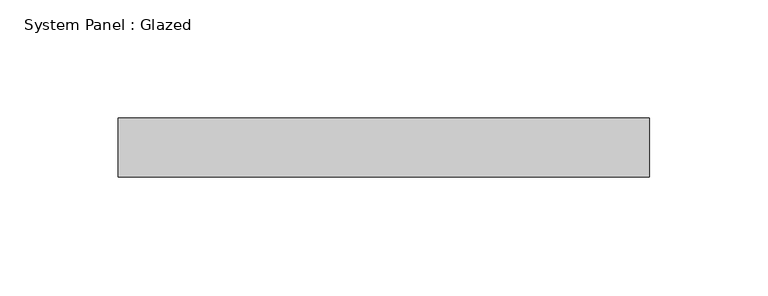
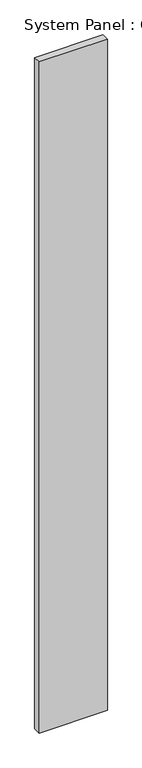
"""IFC4 building model written with IfcOpenShell, lengths in millimetres: plate geometry, System Panel : Glazed."""

from ifc_helpers import new_model, si_unit, origin, origin_with_axes, place, context, project, spatial, polyline, outline, extrude, source, transform, mapped, element, save


def system_panel_glazed_e22c965b(model_context):
    return source(origin(), model_context, "Body", "SweptSolid", [
        extrude(outline(polyline([(112.5, 24.5), (-112.5, 24.5), (-112.5, 49.5), (112.5, 49.5), (112.5, 24.5)])), origin_with_axes(), (0.0, 0.0, 1.0), 2338.4),
    ])


if __name__ == "__main__":
    model = new_model("IFC4")
    model_context = context("Model", 3, world=origin())
    ifc_project = project(units=[si_unit("LENGTHUNIT", "METRE", prefix="MILLI")], contexts=[model_context])
    site = spatial("IfcSite", under=ifc_project)
    building = spatial("IfcBuilding", under=site)
    placement = place(None, origin())
    system_panel_glazed_shape = system_panel_glazed_e22c965b(model_context)
    element("IfcPlate", 1, ObjectType="System Panel : Glazed", at=placement, inside=building, context=model_context, shape_type="MappedRepresentation", body=[
        mapped(system_panel_glazed_shape, transform((0.0, 0.0, 0.0), x_axis=(1.0, 0.0, 0.0), y_axis=(0.0, 1.0, 0.0), z_axis=(0.0, 0.0, 1.0))),
    ])
    save(model, "model.ifc")

# Revit data of these elements
# Type "System Panel : Glazed"
#   Construction Type Id = "GSP4R"
#   Analytic Construction = "1/8 in Pilkington single glazing"
#   Visual Light Transmittance = 0.9
#   Solar Heat Gain Coefficient = 0.86
#   Heat Transfer Coefficient (U) = 6.7069 W/(m²·K)
# Element 1 (IfcPlate, "System Panel : Glazed")
#   Materials on its faces: "Glass"
# Materials
#   "Glass": class "Glass", colour RGB 0 128 192, transparency 0.9, Description = "Soda Lime Glass", Cost = 0
